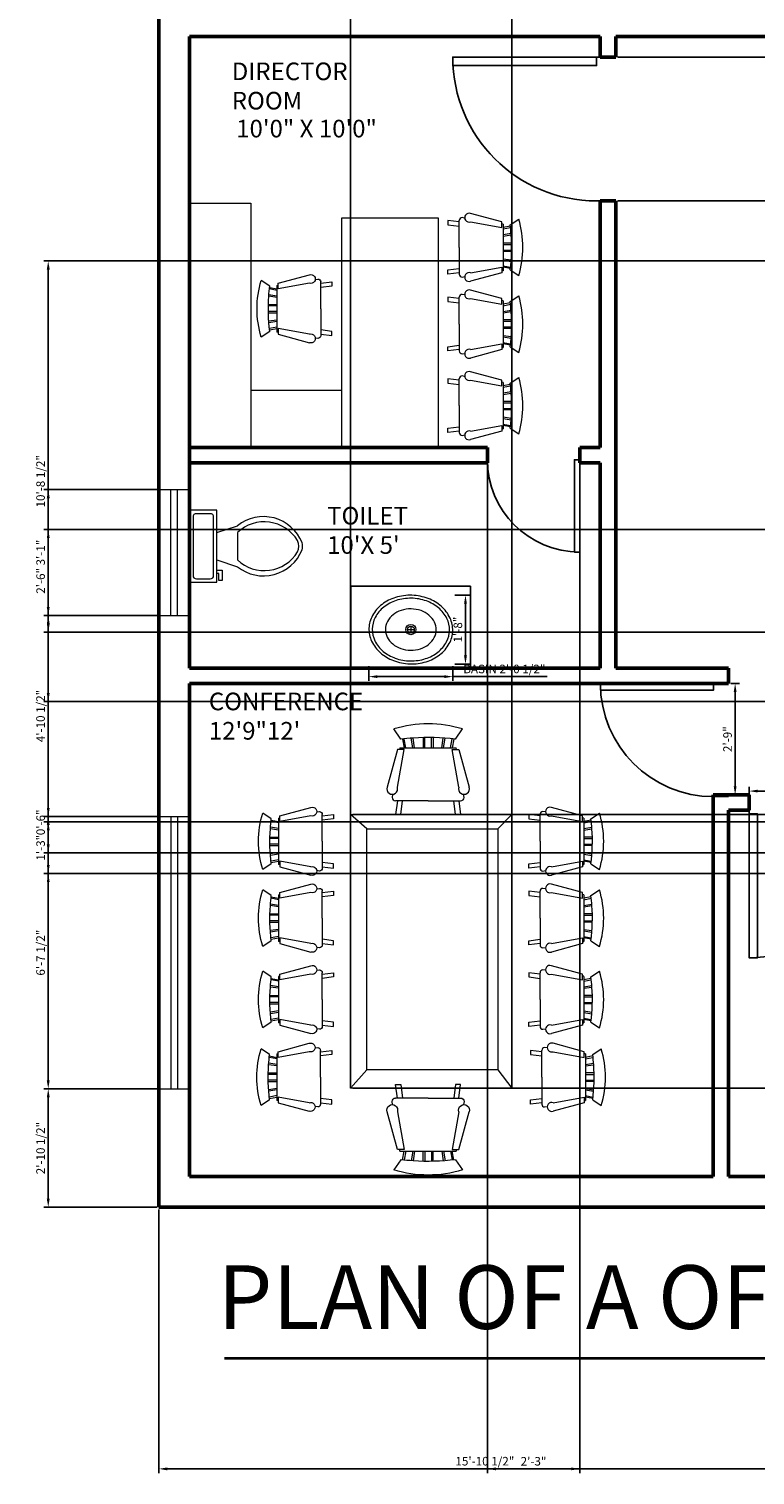
# Model space of a CAD drawing. Units: inches. Extents: x -4852 to -4300, y 4342 to 5059.
# Tile 1 of 4: x -4852 to -4640, y 4342 to 4764. Entities that reach past the tile are written whole.
import ezdxf

# ---------------------------------------------------------------- set-up
doc = ezdxf.new("R2010")
doc.units = ezdxf.units.IN
for name, color, linetype, lineweight in [('A-ANNO-DIMS', 2, 'Continuous', 18), ('A-ANNO-TITL', 7, 'Continuous', 35), ('A-AREA-IDEN', 7, 'Continuous', 18), ('A-DOOR', 4, 'Continuous', 25), ('A-FLOR-CASE', 9, 'Continuous', 25), ('A-FLOR-FIXT', 9, 'Continuous', 18), ('A-FURN', 8, 'Continuous', 18), ('A-GLAZ', 4, 'Continuous', 18), ('A-WALL', 7, 'Continuous', 50)]:
    doc.layers.add(name, color=color, linetype=linetype, lineweight=lineweight)
doc.styles.get("Standard").update_dxf_attribs({"font": 'arial.ttf'})
doc.dimstyles.new('ISO-25', dxfattribs={"dimtxt": 2.5, "dimasz": 2.5, "dimexe": 1.25, "dimexo": 0.625, "dimtad": 1, "dimdec": 0, "dimlunit": 3, "dimtxsty": 'Standard', "dimcen": 2.5, "dimadec": 0, "dimazin": 0, "dimtfac": 1, "dimtdec": 0, "dimtmove": 0, "dimatfit": 3, "dimfxl": 1, "dimarcsym": 0})

# ---------------------------------------------------------------- blocks, each defined once
blk = doc.blocks.new('*U2')
for p, q in [((0, 0), (0, -100)), ((750, 0), (750, -100))]:
    blk.add_line(p, q)
blk.add_lwpolyline([(0, 0), (0, 750), (43.75, 750), (43.75, 0)], close=True)
blk.add_arc((0, 0), 750, 0, 90)
blk = doc.blocks.new('Toilet - top')
for p, q in [((9.5, -6), (9.5, -2)), ((-8, -8.5), (-8, -8)), ((-7, -8), (-7, -9.5)), ((-4, -8), (-6, -14)), ((4, -8), (6, -14)), ((-10, -8.5), (-8, -8.5)), ((-10, -9.5), (-10, -8.5)), ((-7, -9.5), (-10, -9.5)), ((4, -14), (-4, -14))]:
    blk.add_line(p, q)
blk.add_lwpolyline([(10.5, -8), (10.5, 0), (-10.5, 0), (-10.5, -8)], close=True)
for points in [[(-9.5, -2), (-9.5, -6)], [(8.5, -1), (-8.5, -1)], [(-8.5, -7), (8.5, -7)]]:
    blk.add_lwpolyline(points)
for centre, radius, start, end in [((-8.62, -1.88), 0.884, 81.8699, 188.1301), ((8.62, -1.88), 0.884, 351.8699, 98.1301), ((-8.62, -6.12), 0.884, 171.8699, 278.1301), ((8.62, -6.12), 0.884, 261.8699, 8.1301), ((3.52, -21.58), 12.17, 141.4691, 247.9714), ((4.2, -21.82), 11.33, 136.3677, 238.9468), ((-3.52, -21.58), 12.17, 292.0284, 38.5307), ((-4.2, -21.82), 11.33, 301.053, 43.6321), ((0, -27.88), 4, 245.7318, 294.2682), ((0, -29), 4, 254.8605, 285.1395)]:
    blk.add_arc(centre, radius, start, end)
blk = doc.blocks.new('Sink - Oval top')
for p, q in [((-1, 0), (1, 0)), ((0, 1), (0, -1))]:
    blk.add_line(p, q)
for points in [[(-12.23, 0.39, 0.117634), (-11.46, -3.36, 0.104469), (-8.88, -6.8, 0.090016), (-5.08, -9.07, 0.08192), (-0.32, -10.02, 0.08192), (4.49, -9.38, 0.090016), (8.42, -7.36, 0.104469), (11.22, -4.09, 0.117634), (12.23, -0.39, 0.117634), (11.46, 3.36, 0.104469), (8.88, 6.8, 0.090016), (5.08, 9.07, 0.08192), (0.32, 10.02, 0.08192), (-4.49, 9.38, 0.090016), (-8.42, 7.36, 0.104469), (-11.22, 4.09, 0.117634)], [(-11.29, 0.16, 0.118622), (-10.52, -3.25, 0.104678), (-8.07, -6.36, 0.089562), (-4.54, -8.37, 0.081185), (-0.13, -9.15, 0.081185), (4.3, -8.49, 0.089562), (7.89, -6.58, 0.104678), (10.42, -3.55, 0.118622), (11.29, -0.16, 0.118622), (10.52, 3.25, 0.104678), (8.07, 6.36, 0.089562), (4.54, 8.37, 0.081185), (0.13, 9.15, 0.081185), (-4.3, 8.49, 0.089562), (-7.89, 6.58, 0.104678), (-10.42, 3.55, 0.118622)], [(-7.42, 0.08, 0.118283), (-6.91, -2.17, 0.104607), (-5.29, -4.21, 0.089718), (-2.97, -5.53, 0.081436), (-0.07, -6.04, 0.081436), (2.84, -5.59, 0.089718), (5.2, -4.33, 0.104607), (6.86, -2.32, 0.118283), (7.42, -0.08, 0.118283), (6.91, 2.17, 0.104607), (5.29, 4.21, 0.089718), (2.97, 5.53, 0.081436), (0.07, 6.04, 0.081436), (-2.84, 5.59, 0.089718), (-5.2, 4.33, 0.104607), (-6.86, 2.32, 0.118283)]]:
    blk.add_lwpolyline(points, format="xyb", close=True)
for radius in [1.5, 1]:
    blk.add_circle((0, 0), radius)
blk = doc.blocks.new('Chair - Rocking')
for p, q in [((-8, -4.5), (-10, -1.5)), ((-4.5, -7), (-4.96674, -4.19951)), ((-4, -7), (-4.40532, -4.16272)), ((-1.5, -4.05012), (-1.5, -7)), ((-1, -7), (-1, -4.05012)), ((1, -7), (1, -4.04655)), ((1.5, -4.05012), (1.5, -7)), ((4, -7), (4.40187, -4.18694)), ((4.5, -7), (4.96761, -4.19437)), ((8, -4.5), (10, -1.5)), ((-9, -7.5), (-12, -18.49999)), ((-7, -7.5), (-9, -7.5)), ((-9, -18.49999), (-7, -7.5)), ((-8.23428, -6.99939), (-8.3093, -7.47958)), ((-8.23041, -7), (8.23915, -7)), ((-7.5, -4.5), (-7, -7)), ((-6.5, -7), (-7.02225, -4.43)), ((6.5, -7), (7, -4.4057)), ((7.5, -4.5), (7, -7)), ((7, -7.5), (9, -7.5)), ((9, -18.49999), (7, -7.5)), ((8.31071, -7.48854), (8.23449, -7.00073)), ((9, -7.5), (12, -18.49999)), ((-10.36644, -20.64523), (-10.5, -21.49999)), ((10.5, -21.49999), (10.3575, -20.58798)), ((-9, -22.49999), (-9.5, -26.49999)), ((0, -22.49999), (-9.5, -22.49999)), ((-8, -26.49999), (-7.5, -22.49999)), ((0, -22.49999), (9.5, -22.49999)), ((8, -26.49999), (7.5, -22.49999)), ((9, -22.49999), (9.5, -26.49999)), ((-9.5, -26.49999), (-8, -26.49999)), ((9.5, -26.49999), (8, -26.49999))]:
    blk.add_line(p, q)
for centre, radius, start, end in [((0, -34.08333), 34.08333, 72.93847, 107.0615), ((0, -68.25004), 64.25, 93.92211, 97.15267), ((0, -68.25004), 64.25, 82.84733, 93.92211), ((-10.5, -18.99999), 1.58114, 161.5651, 18.43495), ((10.5, -18.99999), 1.58114, 161.5651, 18.43495), ((-9.5, -21.49999), 1, 180, 270), ((9.5, -21.49999), 1, 270, 0)]:
    blk.add_arc(centre, radius, start, end)
blk = doc.blocks.new('*D8')
at = {"layer": 'A-ANNO-DIMS', "color": 0, "lineweight": -2, "transparency": 16777216}
for p, q in [((-4646.77, 4572.88), (-4644.24, 4572.88)), ((-4645.49, 4570.38), (-4645.49, 4542.88)), ((-4646.77, 4540.38), (-4644.24, 4540.38))]:
    blk.add_line(p, q, dxfattribs=at)
at = {"layer": 'A-ANNO-DIMS', "color": 0, "transparency": 16777216}
for points in [[(-4645.91, 4570.38), (-4645.07, 4570.38), (-4645.49, 4572.88)], [(-4645.91, 4542.88), (-4645.07, 4542.88), (-4645.49, 4540.38)]]:
    blk.add_solid(points, dxfattribs=at)
at = {"layer": 'Defpoints', "color": 0, "transparency": 16777216}
for p in [(-4647.4, 4572.88), (-4647.4, 4540.38), (-4645.49, 4540.38)]:
    blk.add_point(p, dxfattribs=at)
at = {"layer": 'A-ANNO-DIMS', "color": 0, "transparency": 16777216, "insert": (-4647.39, 4556.63), "char_height": 2.5, "attachment_point": 5, "rotation": 90}
blk.add_mtext('2\'-9"', dxfattribs=at)
blk = doc.blocks.new('*D9')
at = {"layer": 'A-ANNO-DIMS', "color": 0, "lineweight": -2, "transparency": 16777216}
for p, q in [((-4641.4, 4535.4), (-4641.4, 4542.7)), ((-4599.4, 4536.5), (-4599.4, 4542.7)), ((-4638.9, 4541.45), (-4601.9, 4541.45))]:
    blk.add_line(p, q, dxfattribs=at)
at = {"layer": 'A-ANNO-DIMS', "color": 0, "transparency": 16777216}
for points in [[(-4638.9, 4541.87), (-4638.9, 4541.04), (-4641.4, 4541.45)], [(-4601.9, 4541.87), (-4601.9, 4541.04), (-4599.4, 4541.45)]]:
    blk.add_solid(points, dxfattribs=at)
at = {"layer": 'Defpoints', "color": 0, "transparency": 16777216}
for p in [(-4599.4, 4541.45), (-4641.4, 4534.78), (-4599.4, 4535.88)]:
    blk.add_point(p, dxfattribs=at)
at = {"layer": 'A-ANNO-DIMS', "color": 0, "transparency": 16777216, "insert": (-4620.4, 4543.36), "char_height": 2.5, "attachment_point": 5}
blk.add_mtext('3\'-6"', dxfattribs=at)
blk = doc.blocks.new('*D29')
at = {"layer": 'A-ANNO-DIMS', "color": 0, "lineweight": -2, "transparency": 16777216}
for p, q in [((-4752.52, 4577.95), (-4752.52, 4573.64)), ((-4727.97, 4577.95), (-4727.97, 4573.64)), ((-4750.02, 4574.89), (-4730.47, 4574.89)), ((-4727.97, 4574.89), (-4700.41, 4574.89))]:
    blk.add_line(p, q, dxfattribs=at)
at = {"layer": 'A-ANNO-DIMS', "color": 0, "transparency": 16777216}
for points in [[(-4750.02, 4575.31), (-4750.02, 4574.47), (-4752.52, 4574.89)], [(-4730.47, 4575.31), (-4730.47, 4574.47), (-4727.97, 4574.89)]]:
    blk.add_solid(points, dxfattribs=at)
at = {"layer": 'Defpoints', "color": 0, "transparency": 16777216}
for p in [(-4752.52, 4578.57), (-4727.97, 4578.57), (-4727.97, 4574.89)]:
    blk.add_point(p, dxfattribs=at)
at = {"layer": 'A-ANNO-DIMS', "color": 0, "transparency": 16777216, "insert": (-4712.94, 4576.81), "char_height": 2.5, "attachment_point": 5}
blk.add_mtext('BASIN 2\'-0 1/2"', dxfattribs=at)
blk = doc.blocks.new('*D30')
at = {"layer": 'A-ANNO-DIMS', "color": 0, "lineweight": -2, "transparency": 16777216}
for p, q in [((-4727.35, 4598.71), (-4723.04, 4598.71)), ((-4724.29, 4581.07), (-4724.29, 4596.21)), ((-4727.35, 4578.57), (-4723.04, 4578.57))]:
    blk.add_line(p, q, dxfattribs=at)
at = {"layer": 'A-ANNO-DIMS', "color": 0, "transparency": 16777216}
for points in [[(-4724.71, 4596.21), (-4723.87, 4596.21), (-4724.29, 4598.71)], [(-4724.71, 4581.07), (-4723.87, 4581.07), (-4724.29, 4578.57)]]:
    blk.add_solid(points, dxfattribs=at)
at = {"layer": 'Defpoints', "color": 0, "transparency": 16777216}
for p in [(-4727.97, 4598.71), (-4724.29, 4598.71), (-4727.97, 4578.57)]:
    blk.add_point(p, dxfattribs=at)
at = {"layer": 'A-ANNO-DIMS', "color": 0, "transparency": 16777216, "insert": (-4726.19, 4588.64), "char_height": 2.5, "attachment_point": 5, "rotation": 90}
blk.add_mtext('1\'-8"', dxfattribs=at)
blk = doc.blocks.new('*D46')
at = {"layer": 'A-ANNO-DIMS', "color": 0, "lineweight": -2, "transparency": 16777216}
for p, q in [((-4679.77, 4755.88), (-4300.34, 4755.88)), ((-4301.59, 4716.38), (-4301.59, 4753.38)), ((-4679.77, 4713.88), (-4300.34, 4713.88))]:
    blk.add_line(p, q, dxfattribs=at)
at = {"layer": 'A-ANNO-DIMS', "color": 0, "transparency": 16777216}
for points in [[(-4302.01, 4753.38), (-4301.17, 4753.38), (-4301.59, 4755.88)], [(-4302.01, 4716.38), (-4301.17, 4716.38), (-4301.59, 4713.88)]]:
    blk.add_solid(points, dxfattribs=at)
at = {"layer": 'Defpoints', "color": 0, "transparency": 16777216}
for p in [(-4680.4, 4755.88), (-4301.59, 4755.88), (-4680.4, 4713.88)]:
    blk.add_point(p, dxfattribs=at)
at = {"layer": 'A-ANNO-DIMS', "color": 0, "transparency": 16777216, "insert": (-4303.49, 4734.88), "char_height": 2.5, "attachment_point": 5, "rotation": 90}
blk.add_mtext('3\'-6"', dxfattribs=at)
blk = doc.blocks.new('*D47')
at = {"layer": 'A-ANNO-DIMS', "color": 0, "lineweight": -2, "transparency": 16777216}
for p, q in [((-4717.9, 4636.75), (-4717.9, 4342.18)), ((-4690.9, 4636.75), (-4690.9, 4342.18)), ((-4715.4, 4343.43), (-4693.4, 4343.43))]:
    blk.add_line(p, q, dxfattribs=at)
at = {"layer": 'A-ANNO-DIMS', "color": 0, "transparency": 16777216}
for points in [[(-4715.4, 4343.85), (-4715.4, 4343.01), (-4717.9, 4343.43)], [(-4693.4, 4343.85), (-4693.4, 4343.01), (-4690.9, 4343.43)]]:
    blk.add_solid(points, dxfattribs=at)
at = {"layer": 'Defpoints', "color": 0, "transparency": 16777216}
for p in [(-4717.9, 4637.38), (-4690.9, 4637.38), (-4690.9, 4343.43)]:
    blk.add_point(p, dxfattribs=at)
at = {"layer": 'A-ANNO-DIMS', "color": 0, "transparency": 16777216, "insert": (-4704.4, 4345.33), "char_height": 2.5, "attachment_point": 5}
blk.add_mtext('2\'-3"', dxfattribs=at)
blk = doc.blocks.new('*D48')
at = {"layer": 'A-ANNO-DIMS', "color": 0, "lineweight": -2, "transparency": 16777216}
for p, q in [((-4468.02, 4617.88), (-4847.46, 4617.88)), ((-4846.21, 4590.38), (-4846.21, 4615.38)), ((-4468.02, 4587.88), (-4847.46, 4587.88))]:
    blk.add_line(p, q, dxfattribs=at)
at = {"layer": 'A-ANNO-DIMS', "color": 0, "transparency": 16777216}
for points in [[(-4846.63, 4615.38), (-4845.79, 4615.38), (-4846.21, 4617.88)], [(-4846.63, 4590.38), (-4845.79, 4590.38), (-4846.21, 4587.88)]]:
    blk.add_solid(points, dxfattribs=at)
at = {"layer": 'Defpoints', "color": 0, "transparency": 16777216}
for p in [(-4846.21, 4617.88), (-4467.4, 4617.88), (-4467.4, 4587.88)]:
    blk.add_point(p, dxfattribs=at)
at = {"layer": 'A-ANNO-DIMS', "color": 0, "transparency": 16777216, "insert": (-4848.11, 4602.88), "char_height": 2.5, "attachment_point": 5, "rotation": 90}
blk.add_mtext('2\'-6"', dxfattribs=at)
blk = doc.blocks.new('*D50')
at = {"layer": 'A-ANNO-DIMS', "color": 0, "lineweight": -2, "transparency": 16777216}
for p, q in [((-4814.52, 4454.45), (-4847.46, 4454.45)), ((-4846.21, 4422.38), (-4846.21, 4451.95)), ((-4814.52, 4419.88), (-4847.46, 4419.88))]:
    blk.add_line(p, q, dxfattribs=at)
at = {"layer": 'A-ANNO-DIMS', "color": 0, "transparency": 16777216}
for points in [[(-4846.63, 4451.95), (-4845.79, 4451.95), (-4846.21, 4454.45)], [(-4846.63, 4422.38), (-4845.79, 4422.38), (-4846.21, 4419.88)]]:
    blk.add_solid(points, dxfattribs=at)
at = {"layer": 'Defpoints', "color": 0, "transparency": 16777216}
for p in [(-4846.21, 4454.45), (-4813.9, 4454.45), (-4813.9, 4419.88)]:
    blk.add_point(p, dxfattribs=at)
at = {"layer": 'A-ANNO-DIMS', "color": 0, "transparency": 16777216, "insert": (-4848.13, 4437.16), "char_height": 2.5, "attachment_point": 5, "rotation": 90}
blk.add_mtext('2\'-10 1/2"', dxfattribs=at)
blk = doc.blocks.new('*D51')
at = {"layer": 'A-ANNO-DIMS', "color": 0, "lineweight": -2, "transparency": 16777216}
for p, q in [((-4814.52, 4534.05), (-4847.46, 4534.05)), ((-4846.21, 4456.95), (-4846.21, 4531.55)), ((-4814.52, 4454.45), (-4847.46, 4454.45))]:
    blk.add_line(p, q, dxfattribs=at)
at = {"layer": 'A-ANNO-DIMS', "color": 0, "transparency": 16777216}
for points in [[(-4846.63, 4531.55), (-4845.79, 4531.55), (-4846.21, 4534.05)], [(-4846.63, 4456.95), (-4845.79, 4456.95), (-4846.21, 4454.45)]]:
    blk.add_solid(points, dxfattribs=at)
at = {"layer": 'Defpoints', "color": 0, "transparency": 16777216}
for p in [(-4846.21, 4534.05), (-4813.9, 4534.05), (-4813.9, 4454.45)]:
    blk.add_point(p, dxfattribs=at)
at = {"layer": 'A-ANNO-DIMS', "color": 0, "transparency": 16777216, "insert": (-4848.13, 4494.25), "char_height": 2.5, "attachment_point": 5, "rotation": 90}
blk.add_mtext('6\'-7 1/2"', dxfattribs=at)
blk = doc.blocks.new('*D52')
at = {"layer": 'A-ANNO-DIMS', "color": 0, "lineweight": -2, "transparency": 16777216}
for p, q in [((-4814.52, 4592.74), (-4847.46, 4592.74)), ((-4846.21, 4536.55), (-4846.21, 4590.24)), ((-4814.52, 4534.05), (-4847.46, 4534.05))]:
    blk.add_line(p, q, dxfattribs=at)
at = {"layer": 'A-ANNO-DIMS', "color": 0, "transparency": 16777216}
for points in [[(-4846.63, 4590.24), (-4845.79, 4590.24), (-4846.21, 4592.74)], [(-4846.63, 4536.55), (-4845.79, 4536.55), (-4846.21, 4534.05)]]:
    blk.add_solid(points, dxfattribs=at)
at = {"layer": 'Defpoints', "color": 0, "transparency": 16777216}
for p in [(-4846.21, 4592.74), (-4813.9, 4592.74), (-4813.9, 4534.05)]:
    blk.add_point(p, dxfattribs=at)
at = {"layer": 'A-ANNO-DIMS', "color": 0, "transparency": 16777216, "insert": (-4848.13, 4563.4), "char_height": 2.5, "attachment_point": 5, "rotation": 90}
blk.add_mtext('4\'-10 1/2"', dxfattribs=at)
blk = doc.blocks.new('*D53')
at = {"layer": 'A-ANNO-DIMS', "color": 0, "lineweight": -2, "transparency": 16777216}
for p, q in [((-4814.52, 4629.53), (-4847.46, 4629.53)), ((-4846.21, 4595.24), (-4846.21, 4627.03)), ((-4814.52, 4592.74), (-4847.46, 4592.74))]:
    blk.add_line(p, q, dxfattribs=at)
at = {"layer": 'A-ANNO-DIMS', "color": 0, "transparency": 16777216}
for points in [[(-4846.63, 4627.03), (-4845.79, 4627.03), (-4846.21, 4629.53)], [(-4846.63, 4595.24), (-4845.79, 4595.24), (-4846.21, 4592.74)]]:
    blk.add_solid(points, dxfattribs=at)
at = {"layer": 'Defpoints', "color": 0, "transparency": 16777216}
for p in [(-4846.21, 4629.53), (-4813.9, 4629.53), (-4813.9, 4592.74)]:
    blk.add_point(p, dxfattribs=at)
at = {"layer": 'A-ANNO-DIMS', "color": 0, "transparency": 16777216, "insert": (-4848.11, 4611.14), "char_height": 2.5, "attachment_point": 5, "rotation": 90}
blk.add_mtext('3\'-1"', dxfattribs=at)
blk = doc.blocks.new('*D54')
at = {"layer": 'A-ANNO-DIMS', "color": 0, "lineweight": -2, "transparency": 16777216}
for p, q in [((-4813.9, 4419.25), (-4813.9, 4342.18)), ((-4623.35, 4419.25), (-4623.35, 4342.18)), ((-4811.4, 4343.43), (-4625.85, 4343.43))]:
    blk.add_line(p, q, dxfattribs=at)
at = {"layer": 'A-ANNO-DIMS', "color": 0, "transparency": 16777216}
for points in [[(-4811.4, 4343.85), (-4811.4, 4343.01), (-4813.9, 4343.43)], [(-4625.85, 4343.85), (-4625.85, 4343.01), (-4623.35, 4343.43)]]:
    blk.add_solid(points, dxfattribs=at)
at = {"layer": 'Defpoints', "color": 0, "transparency": 16777216}
for p in [(-4813.9, 4419.88), (-4623.35, 4419.88), (-4623.35, 4343.43)]:
    blk.add_point(p, dxfattribs=at)
at = {"layer": 'A-ANNO-DIMS', "color": 0, "transparency": 16777216, "insert": (-4718.62, 4345.35), "char_height": 2.5, "attachment_point": 5}
blk.add_mtext('15\'-10 1/2"', dxfattribs=at)
blk = doc.blocks.new('*D61')
at = {"layer": 'A-ANNO-DIMS', "color": 0, "lineweight": -2, "transparency": 16777216}
for p, q in [((-4635.56, 4696.34), (-4847.46, 4696.34)), ((-4846.21, 4693.84), (-4846.21, 4570.1)), ((-4607.33, 4567.6), (-4847.46, 4567.6))]:
    blk.add_line(p, q, dxfattribs=at)
at = {"layer": 'A-ANNO-DIMS', "color": 0, "transparency": 16777216}
for points in [[(-4846.63, 4693.84), (-4845.79, 4693.84), (-4846.21, 4696.34)], [(-4846.63, 4570.1), (-4845.79, 4570.1), (-4846.21, 4567.6)]]:
    blk.add_solid(points, dxfattribs=at)
at = {"layer": 'Defpoints', "color": 0, "transparency": 16777216}
for p in [(-4634.93, 4696.34), (-4846.21, 4567.6), (-4606.71, 4567.6)]:
    blk.add_point(p, dxfattribs=at)
at = {"layer": 'A-ANNO-DIMS', "color": 0, "transparency": 16777216, "insert": (-4848.13, 4631.97), "char_height": 2.5, "attachment_point": 5, "rotation": 90}
blk.add_mtext('10\'-8 1/2"', dxfattribs=at)
blk = doc.blocks.new('*D62')
at = {"layer": 'A-ANNO-DIMS', "color": 0, "lineweight": -2, "transparency": 16777216}
for p, q in [((-4757.87, 4455.31), (-4757.87, 5054.94)), ((-4755.37, 5053.69), (-4713.26, 5053.69)), ((-4710.76, 4455.31), (-4710.76, 5054.94))]:
    blk.add_line(p, q, dxfattribs=at)
at = {"layer": 'A-ANNO-DIMS', "color": 0, "transparency": 16777216}
for points in [[(-4755.37, 5054.11), (-4755.37, 5053.27), (-4757.87, 5053.69)], [(-4713.26, 5054.11), (-4713.26, 5053.27), (-4710.76, 5053.69)]]:
    blk.add_solid(points, dxfattribs=at)
at = {"layer": 'Defpoints', "color": 0, "transparency": 16777216}
for p in [(-4710.76, 5053.69), (-4757.87, 4454.69), (-4710.76, 4454.69)]:
    blk.add_point(p, dxfattribs=at)
at = {"layer": 'A-ANNO-DIMS', "color": 0, "transparency": 16777216, "insert": (-4734.32, 5055.59), "char_height": 2.5, "attachment_point": 5}
blk.add_mtext('3\'-11"', dxfattribs=at)
blk = doc.blocks.new('*D63')
at = {"layer": 'A-ANNO-DIMS', "color": 0, "lineweight": -2, "transparency": 16777216}
for p, q in [((-4757.25, 4534.6), (-4300.34, 4534.6)), ((-4301.59, 4457.19), (-4301.59, 4532.1)), ((-4757.25, 4454.69), (-4300.34, 4454.69))]:
    blk.add_line(p, q, dxfattribs=at)
at = {"layer": 'A-ANNO-DIMS', "color": 0, "transparency": 16777216}
for points in [[(-4302.01, 4532.1), (-4301.17, 4532.1), (-4301.59, 4534.6)], [(-4302.01, 4457.19), (-4301.17, 4457.19), (-4301.59, 4454.69)]]:
    blk.add_solid(points, dxfattribs=at)
at = {"layer": 'Defpoints', "color": 0, "transparency": 16777216}
for p in [(-4757.87, 4534.6), (-4301.59, 4534.6), (-4757.87, 4454.69)]:
    blk.add_point(p, dxfattribs=at)
at = {"layer": 'A-ANNO-DIMS', "color": 0, "transparency": 16777216, "insert": (-4303.49, 4494.64), "char_height": 2.5, "attachment_point": 5, "rotation": 90}
blk.add_mtext('6\'-8"', dxfattribs=at)
blk = doc.blocks.new('*D64')
at = {"layer": 'A-ANNO-DIMS', "color": 0, "lineweight": -2, "transparency": 16777216}
for p, q in [((-4846.21, 4525.88), (-4846.21, 4536.27)), ((-4463.52, 4523.38), (-4847.46, 4523.38)), ((-4846.21, 4517.38), (-4846.21, 4523.38)), ((-4463.52, 4517.38), (-4847.46, 4517.38)), ((-4846.21, 4514.88), (-4846.21, 4512.38))]:
    blk.add_line(p, q, dxfattribs=at)
at = {"layer": 'A-ANNO-DIMS', "color": 0, "transparency": 16777216}
for points in [[(-4846.63, 4525.88), (-4845.79, 4525.88), (-4846.21, 4523.38)], [(-4846.63, 4514.88), (-4845.79, 4514.88), (-4846.21, 4517.38)]]:
    blk.add_solid(points, dxfattribs=at)
at = {"layer": 'Defpoints', "color": 0, "transparency": 16777216}
for p in [(-4846.21, 4523.38), (-4462.9, 4523.38), (-4462.9, 4517.38)]:
    blk.add_point(p, dxfattribs=at)
at = {"layer": 'A-ANNO-DIMS', "color": 0, "transparency": 16777216, "insert": (-4848.11, 4532.33), "char_height": 2.5, "attachment_point": 5, "rotation": 90}
blk.add_mtext('0\'-6"', dxfattribs=at)
blk = doc.blocks.new('*D65')
at = {"layer": 'A-ANNO-DIMS', "color": 0, "lineweight": -2, "transparency": 16777216}
for p, q in [((-4367.52, 4532.45), (-4847.46, 4532.45)), ((-4846.21, 4519.88), (-4846.21, 4529.95)), ((-4367.52, 4517.38), (-4847.46, 4517.38))]:
    blk.add_line(p, q, dxfattribs=at)
at = {"layer": 'A-ANNO-DIMS', "color": 0, "transparency": 16777216}
for points in [[(-4846.63, 4529.95), (-4845.79, 4529.95), (-4846.21, 4532.45)], [(-4846.63, 4519.88), (-4845.79, 4519.88), (-4846.21, 4517.38)]]:
    blk.add_solid(points, dxfattribs=at)
at = {"layer": 'Defpoints', "color": 0, "transparency": 16777216}
for p in [(-4846.21, 4532.45), (-4366.9, 4532.45), (-4366.9, 4517.38)]:
    blk.add_point(p, dxfattribs=at)
at = {"layer": 'A-ANNO-DIMS', "color": 0, "transparency": 16777216, "insert": (-4848.11, 4524.92), "char_height": 2.5, "attachment_point": 5, "rotation": 90}
blk.add_mtext('1\'-3"', dxfattribs=at)

msp = doc.modelspace()

# ---------------------------------------------------------------- linework, layer by layer
at = {"layer": 'A-ANNO-TITL'}
msp.add_line((-4794.71, 4375.74), (-4430.92, 4375.74), dxfattribs=at)
at = {"layer": 'A-FLOR-CASE'}
for p, q in [((-4722.79, 4601.31), (-4757.76, 4601.31)), ((-4757.76, 4601.31), (-4757.76, 4577.38)), ((-4722.79, 4577.38), (-4722.79, 4601.31))]:
    msp.add_line(p, q, dxfattribs=at)
at = {"layer": 'A-FURN'}
for p, q in [((-4787.03, 4658.56), (-4760.39, 4658.56)), ((-4753.09, 4530.39), (-4757.87, 4534.6)), ((-4714.87, 4530.39), (-4710.76, 4534.6)), ((-4753.09, 4459.98), (-4757.87, 4454.69)), ((-4714.87, 4459.98), (-4710.76, 4454.69))]:
    msp.add_line(p, q, dxfattribs=at)
for points in [[(-4787.03, 4641.88), (-4804.9, 4641.88), (-4804.9, 4713.21), (-4787.03, 4713.21)], [(-4760.39, 4708.93), (-4732.31, 4708.93), (-4732.31, 4641.88), (-4760.39, 4641.88)], [(-4757.87, 4534.6), (-4710.76, 4534.6), (-4710.76, 4454.69), (-4757.87, 4454.69)], [(-4753.09, 4530.39), (-4714.87, 4530.39), (-4714.87, 4459.98), (-4753.09, 4459.98)]]:
    msp.add_lwpolyline(points, close=True, dxfattribs=at)
at = {"layer": 'A-GLAZ'}
for p, q in [((-4813.9, 4629.53), (-4804.9, 4629.53)), ((-4810.4, 4592.74), (-4810.4, 4629.53)), ((-4808.4, 4592.74), (-4808.4, 4629.53)), ((-4813.9, 4592.74), (-4804.9, 4592.74)), ((-4813.9, 4534.05), (-4804.9, 4534.05)), ((-4810.4, 4534.05), (-4810.4, 4454.58)), ((-4808.4, 4534.05), (-4808.4, 4454.58)), ((-4813.9, 4454.45), (-4804.9, 4454.45))]:
    msp.add_line(p, q, dxfattribs=at)
at = {"layer": 'A-WALL'}
for p, q in [((-4813.9, 4907.38), (-4813.9, 4419.88)), ((-4804.9, 4761.88), (-4684.9, 4761.88)), ((-4804.9, 4761.88), (-4804.9, 4577.38)), ((-4684.9, 4761.88), (-4684.9, 4755.88)), ((-4680.4, 4761.88), (-4680.4, 4755.88)), ((-4680.4, 4761.88), (-4533.4, 4761.88)), ((-4684.9, 4755.88), (-4680.4, 4755.88)), ((-4684.9, 4713.88), (-4680.4, 4713.88)), ((-4684.9, 4713.88), (-4684.9, 4641.88)), ((-4680.4, 4713.88), (-4680.4, 4577.38)), ((-4804.9, 4641.88), (-4717.9, 4641.88)), ((-4717.9, 4637.38), (-4717.9, 4641.88)), ((-4690.9, 4637.38), (-4690.9, 4641.88)), ((-4690.9, 4641.88), (-4684.9, 4641.88)), ((-4804.9, 4637.38), (-4717.9, 4637.38)), ((-4690.9, 4637.38), (-4684.9, 4637.38)), ((-4684.9, 4637.38), (-4684.9, 4577.38)), ((-4804.9, 4577.38), (-4684.9, 4577.38)), ((-4680.4, 4577.38), (-4647.4, 4577.38)), ((-4647.4, 4577.38), (-4647.4, 4572.88)), ((-4804.9, 4572.88), (-4647.4, 4572.88)), ((-4804.9, 4572.88), (-4804.9, 4428.88)), ((-4651.9, 4540.38), (-4641.4, 4540.38)), ((-4651.9, 4540.38), (-4651.9, 4428.88)), ((-4641.4, 4540.38), (-4641.4, 4535.88)), ((-4647.4, 4535.88), (-4641.4, 4535.88)), ((-4647.4, 4535.88), (-4647.4, 4428.88)), ((-4804.9, 4428.88), (-4651.9, 4428.88)), ((-4647.4, 4428.88), (-4333.9, 4428.88)), ((-4813.9, 4419.88), (-4333.9, 4419.88))]:
    msp.add_line(p, q, dxfattribs=at)

# ---------------------------------------------------------------- block references
at = {"layer": 'A-DOOR'}
for p, xscale, yscale, zscale, rotation in [((-4686, 4755.88), -0.0560000000000001, 0.0560000000000001, 0.0560000000000001, 90), ((-4690.9, 4638.28), 0.0359999999999999, 0.0359999999999999, 0.0359999999999999, 180), ((-4651.81, 4572.88), -0.0440656076524333, 0.0440656076524333, 0.0440656076524333, 90), ((-4641.4, 4534.78), -0.0559999999999998, 0.0559999999999998, 0.0559999999999998, 180)]:
    msp.add_blockref('*U2', p, dxfattribs=dict(at, xscale=xscale, yscale=yscale, zscale=zscale, rotation=rotation))
at = {"layer": 'A-FLOR-FIXT', "rotation": 90}
msp.add_blockref('Toilet - top', (-4804.9, 4612.99), dxfattribs=at)
at = {"layer": 'A-FLOR-FIXT'}
msp.add_blockref('Sink - Oval top', (-4740.25, 4588.64), dxfattribs=at)
at = {"layer": 'A-FURN', "yscale": 0.8265392436159728, "zscale": 0.8265392436159728}
for p, xscale, rotation in [((-4707.5, 4700.31), 0.8265392436159728, 270), ((-4785.2, 4682.38), -0.8265392436159728, 90), ((-4707.5, 4677.89), 0.8265392436159728, 270), ((-4707.5, 4654.06), 0.8265392436159728, 270), ((-4784.74, 4526.78), -0.8265392436159728, 90), ((-4683.9, 4526.78), 0.8265392436159728, 270), ((-4784.74, 4504.35), -0.8265392436159728, 90), ((-4683.9, 4504.35), 0.8265392436159728, 270), ((-4784.74, 4480.53), -0.8265392436159728, 90), ((-4683.9, 4480.53), 0.8265392436159728, 270), ((-4785.24, 4457.86), -0.8265392436159728, 90), ((-4683.39, 4457.86), 0.8265392436159728, 270)]:
    msp.add_blockref('Chair - Rocking', p, dxfattribs=dict(at, xscale=xscale, rotation=rotation))
at = {"layer": 'A-FURN'}
msp.add_blockref('Chair - Rocking', (-4735.2, 4561.1), dxfattribs=at)
at = {"layer": 'A-FURN', "xscale": -1, "rotation": 180}
msp.add_blockref('Chair - Rocking', (-4735.2, 4429.27), dxfattribs=at)

# ---------------------------------------------------------------- texts
at = {"layer": 'A-ANNO-TITL'}
msp.add_text('PLAN OF A OFFICE BUILDING ', height=18.5695, dxfattribs=at).set_placement((-4796.74, 4384.34))
at = {"layer": 'A-AREA-IDEN'}
for s, height, p in [('DIRECTOR', 5.149, (-4792.58, 4749.16)), ('ROOM', 5.149, (-4792.58, 4740.59)), ('10\'0" X 10\'0"', 5.1489, (-4791.29, 4732.43)), ('TOILET', 5.149, (-4764.72, 4619.33)), ("10'X 5'", 5.149, (-4764.72, 4610.77)), ('CONFERENCE', 5.149, (-4799.28, 4565.07)), ('12\'9"12\'', 5.149, (-4799.28, 4556.5))]:
    msp.add_text(s, height=height, dxfattribs=at).set_placement(p)

# ---------------------------------------------------------------- dimensions: what is measured, and where the dimension line sits
at = {"layer": 'A-ANNO-DIMS'}
for base, p1, p2, override, picture, middle in [((-4710.76, 5053.69), (-4757.87, 4454.69), (-4710.76, 4454.69), {"dimdec": 1, "dimlfac": 1, "dimrnd": 0, "dimzin": 1, "dimdsep": 46, "dimlunit": 4, "dimfrac": 2}, '*D62', (-4734.32, 5055.59)), ((-4690.9, 4343.43), (-4717.9, 4637.38), (-4690.9, 4637.38), {"dimdec": 1, "dimlfac": 1, "dimrnd": 0, "dimzin": 1, "dimdsep": 46, "dimlunit": 4, "dimfrac": 2}, '*D47', (-4704.4, 4345.33)), ((-4599.4, 4541.45), (-4641.4, 4534.78), (-4599.4, 4535.88), {"dimclrd": 0, "dimclre": 0, "dimclrt": 0}, '*D9', (-4620.4, 4543.36)), ((-4623.3478, 4343.4305), (-4813.8994, 4419.8793), (-4623.3478, 4419.8793), {"dimdec": 1, "dimlfac": 1, "dimrnd": 0, "dimzin": 1, "dimdsep": 46, "dimlunit": 4, "dimfrac": 2}, '*D54', (-4718.6236, 4345.3482))]:
    dim = msp.add_linear_dim(base=base, p1=p1, p2=p2, dimstyle='ISO-25', override=override, dxfattribs=at)
    dim.commit()
    dim.dimension.update_dxf_attribs({"geometry": picture, "text_midpoint": middle})
for base, p1, p2, override, picture, middle in [((-4301.59, 4755.88), (-4680.4, 4713.88), (-4680.4, 4755.88), {"dimdec": 1, "dimlfac": 1, "dimrnd": 0, "dimzin": 1, "dimdsep": 46, "dimlunit": 4, "dimfrac": 2}, '*D46', (-4303.49, 4734.88)), ((-4846.21, 4567.6), (-4634.93, 4696.34), (-4606.71, 4567.6), {"dimdec": 1, "dimlfac": 1, "dimrnd": 0, "dimzin": 1, "dimdsep": 46, "dimlunit": 4, "dimfrac": 2}, '*D61', (-4848.13, 4631.97)), ((-4846.21, 4629.53), (-4813.9, 4592.74), (-4813.9, 4629.53), {"dimdec": 1, "dimlfac": 1, "dimrnd": 0, "dimzin": 1, "dimdsep": 46, "dimlunit": 4, "dimfrac": 2}, '*D53', (-4848.11, 4611.14)), ((-4846.21, 4617.88), (-4467.4, 4587.88), (-4467.4, 4617.88), {"dimdec": 1, "dimlfac": 1, "dimrnd": 0, "dimzin": 1, "dimdsep": 46, "dimlunit": 4, "dimfrac": 2}, '*D48', (-4848.11, 4602.88)), ((-4724.29, 4598.71), (-4727.97, 4578.57), (-4727.97, 4598.71), {"dimdec": 1, "dimlfac": 1, "dimrnd": 0, "dimzin": 1, "dimdsep": 46, "dimlunit": 4, "dimfrac": 2}, '*D30', (-4726.19, 4588.64)), ((-4846.21, 4592.74), (-4813.9, 4534.05), (-4813.9, 4592.74), {"dimdec": 1, "dimlfac": 1, "dimrnd": 0, "dimzin": 1, "dimdsep": 46, "dimlunit": 4, "dimfrac": 2}, '*D52', (-4848.13, 4563.4)), ((-4645.49015464, 4540.37928057), (-4647.39935985, 4572.87928057), (-4647.39935985, 4540.37928057), {"dimclrd": 0, "dimclre": 0, "dimclrt": 0}, '*D8', (-4647.39158711, 4556.62928057)), ((-4846.21, 4534.05), (-4813.9, 4454.45), (-4813.9, 4534.05), {"dimdec": 1, "dimlfac": 1, "dimrnd": 0, "dimzin": 1, "dimdsep": 46, "dimlunit": 4, "dimfrac": 2}, '*D51', (-4848.13, 4494.25)), ((-4846.21, 4523.38), (-4462.9, 4517.38), (-4462.9, 4523.38), {"dimdec": 1, "dimlfac": 1, "dimrnd": 0, "dimzin": 1, "dimdsep": 46, "dimlunit": 4, "dimfrac": 2}, '*D64', (-4848.11, 4532.33)), ((-4301.59, 4534.6), (-4757.87, 4454.69), (-4757.87, 4534.6), {"dimdec": 1, "dimlfac": 1, "dimrnd": 0, "dimzin": 1, "dimdsep": 46, "dimlunit": 4, "dimfrac": 2}, '*D63', (-4303.49, 4494.64)), ((-4846.21, 4532.45), (-4366.9, 4517.38), (-4366.9, 4532.45), {"dimdec": 1, "dimlfac": 1, "dimrnd": 0, "dimzin": 1, "dimdsep": 46, "dimlunit": 4, "dimfrac": 2}, '*D65', (-4848.11, 4524.92)), ((-4846.21, 4454.45), (-4813.9, 4419.88), (-4813.9, 4454.45), {"dimdec": 1, "dimlfac": 1, "dimrnd": 0, "dimzin": 1, "dimdsep": 46, "dimlunit": 4, "dimfrac": 2}, '*D50', (-4848.13, 4437.16))]:
    dim = msp.add_linear_dim(base=base, p1=p1, p2=p2, angle=90, dimstyle='ISO-25', override=override, dxfattribs=at)
    dim.commit()
    dim.dimension.update_dxf_attribs({"geometry": picture, "text_midpoint": middle})
dim = msp.add_linear_dim(base=(-4727.9728, 4574.8894), p1=(-4752.5237, 4578.572), p2=(-4727.9728, 4578.572), text='BASIN <>', dimstyle='ISO-25', override={"dimdec": 1, "dimlfac": 1, "dimrnd": 0, "dimzin": 1, "dimdsep": 46, "dimlunit": 4, "dimfrac": 2}, dxfattribs=at)
dim.commit()
dim.dimension.update_dxf_attribs({"geometry": '*D29', "text_midpoint": (-4712.9421, 4576.807)})

doc.saveas('drawing.dxf')
